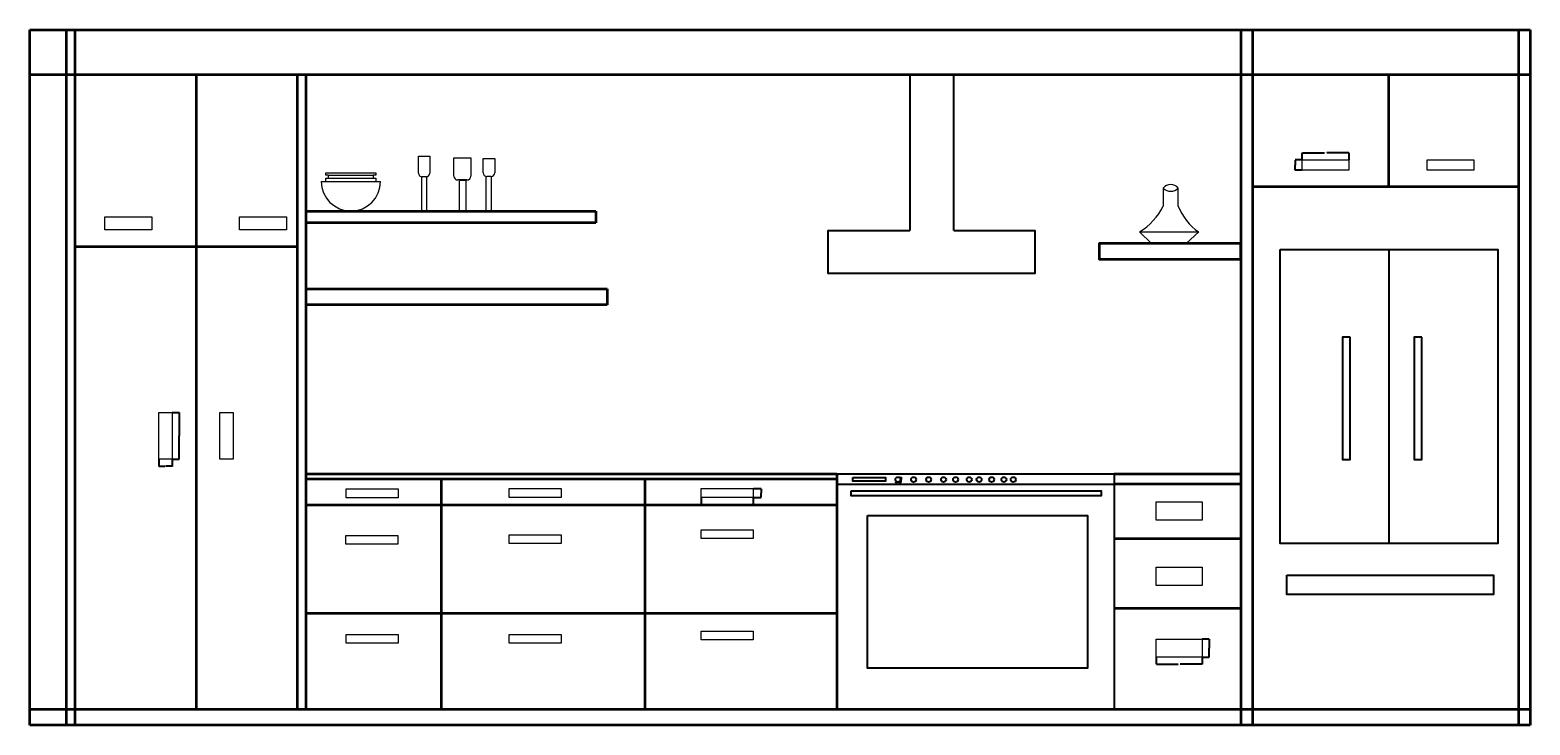
# Model space of a CAD drawing. Units: millimetres. Extents: x 3194 to 5786, y 875 to 2077.
import ezdxf

# ---------------------------------------------------------------- set-up
doc = ezdxf.new("R2010")
doc.units = ezdxf.units.MM
for name, color, linetype, lineweight in [('A-ANNO-DIMS', 2, 'Continuous', 18), ('A-ELEV', 7, 'Continuous', 35), ('A-ELEV-HRDW', 8, 'Continuous', 18), ('A-EQPM', 4, 'Continuous', 25), ('A-FURN', 9, 'Continuous', 18)]:
    doc.layers.add(name, color=color, linetype=linetype, lineweight=lineweight)
doc.styles.get("Standard").update_dxf_attribs({"font": 'arial.ttf'})
doc.dimstyles.get("Standard").update_dxf_attribs({"dimtxt": 0.18, "dimasz": 0.18, "dimexe": 0.18, "dimexo": 0.0625, "dimgap": 0.09, "dimtad": 0, "dimtih": 1, "dimtoh": 1, "dimdec": 4, "dimzin": 0, "dimdsep": 46, "dimtxsty": 'Standard', "dimcen": 0.09, "dimadec": 0, "dimazin": 0, "dimtfac": 1, "dimtdec": 4, "dimtofl": 0, "dimtmove": 0, "dimatfit": 3, "dimfxl": 1, "dimtolj": 1, "dimtzin": 0, "dimarcsym": 0})

# ---------------------------------------------------------------- blocks, each defined once
blk = doc.blocks.new('KNOB-RANGE')
blk.add_circle((4.3, 4.3), 4.31)
blk = doc.blocks.new('PULL-DRAWER-90')
blk.add_lwpolyline([(0, 15.2), (90, 15.2), (90, 0), (0, 0)], close=True)
blk = doc.blocks.new('PULL-DOOR-80')
blk.add_lwpolyline([(0, 81.1), (22.9, 81.1), (22.9, 0), (0, 0)], close=True)
blk = doc.blocks.new('PULL-DRAWER-80')
blk.add_lwpolyline([(0, 31.7), (79.4, 31.7), (79.4, 0), (0, 0)], close=True)
blk = doc.blocks.new('PULL-WALLCAB-80')
blk.add_lwpolyline([(0, 18), (80.8, 18), (80.8, 0), (0, 0)], close=True)
blk = doc.blocks.new('*D6')
at = {"layer": 'A-ANNO-DIMS', "color": 0, "lineweight": -2, "transparency": 16777216}
for p, q in [((4689.7, 1295.1), (4689.7, 1293.7)), ((4689.8, 1293.9), (4692.6, 1293.9)), ((4698.1, 1293.9), (4695.3, 1293.9)), ((4698.3, 1295.1), (4698.3, 1293.7))]:
    blk.add_line(p, q, dxfattribs=at)
at = {"layer": 'A-ANNO-DIMS', "color": 0, "transparency": 16777216}
for points in [[(4689.8, 1293.9), (4689.8, 1293.8), (4689.7, 1293.9)], [(4698.1, 1293.9), (4698.1, 1293.8), (4698.3, 1293.9)]]:
    blk.add_solid(points, dxfattribs=at)
at = {"layer": 'Defpoints', "color": 0, "transparency": 16777216}
for p in [(4689.7, 1295.2), (4698.3, 1295.2), (4698.3, 1293.9)]:
    blk.add_point(p, dxfattribs=at)
at = {"layer": 'A-ANNO-DIMS', "color": 0, "transparency": 16777216, "insert": (4694, 1293.9), "char_height": 0.18, "attachment_point": 5}
blk.add_mtext('\\A1;RANGE KNOB 9 TYP.', dxfattribs=at)
blk = doc.blocks.new('*D7')
at = {"layer": 'A-ANNO-DIMS', "color": 0, "lineweight": -2, "transparency": 16777216}
for p, q in [((4698.3, 1303.8), (4699.8, 1303.8)), ((4699.6, 1303.6), (4699.6, 1299.6)), ((4699.6, 1295.3), (4699.6, 1299.3)), ((4698.3, 1295.2), (4699.8, 1295.2))]:
    blk.add_line(p, q, dxfattribs=at)
at = {"layer": 'A-ANNO-DIMS', "color": 0, "transparency": 16777216}
for points in [[(4699.5, 1303.6), (4699.6, 1303.6), (4699.6, 1303.8)], [(4699.5, 1295.3), (4699.6, 1295.3), (4699.6, 1295.2)]]:
    blk.add_solid(points, dxfattribs=at)
at = {"layer": 'Defpoints', "color": 0, "transparency": 16777216}
for p in [(4698.3, 1303.8), (4699.6, 1303.8), (4698.3, 1295.2)]:
    blk.add_point(p, dxfattribs=at)
at = {"layer": 'A-ANNO-DIMS', "color": 0, "transparency": 16777216, "insert": (4699.6, 1299.5), "char_height": 0.18, "attachment_point": 5}
blk.add_mtext('\\A1;9 TYP.', dxfattribs=at)
blk = doc.blocks.new('*D8')
at = {"layer": 'A-ANNO-DIMS', "color": 0, "lineweight": -2, "transparency": 16777216}
for p, q in [((4354.1, 1268.6), (4354.1, 1254.9)), ((4354.3, 1255.1), (4397.6, 1255.1)), ((4443.9, 1255.1), (4400.6, 1255.1)), ((4444.1, 1268.6), (4444.1, 1254.9))]:
    blk.add_line(p, q, dxfattribs=at)
at = {"layer": 'A-ANNO-DIMS', "color": 0, "transparency": 16777216}
for points in [[(4354.3, 1255.2), (4354.3, 1255.1), (4354.1, 1255.1)], [(4443.9, 1255.2), (4443.9, 1255.1), (4444.1, 1255.1)]]:
    blk.add_solid(points, dxfattribs=at)
at = {"layer": 'Defpoints', "color": 0, "transparency": 16777216}
for p in [(4354.1, 1268.6), (4444.1, 1268.6), (4444.1, 1255.1)]:
    blk.add_point(p, dxfattribs=at)
at = {"layer": 'A-ANNO-DIMS', "color": 0, "transparency": 16777216, "insert": (4399.1, 1255.1), "char_height": 0.18, "attachment_point": 5}
blk.add_mtext('\\A1;DRAWER PULL 90 TYP.', dxfattribs=at)
blk = doc.blocks.new('*D9')
at = {"layer": 'A-ANNO-DIMS', "color": 0, "lineweight": -2, "transparency": 16777216}
for p, q in [((4444.2, 1283.9), (4457.8, 1283.9)), ((4457.6, 1283.7), (4457.6, 1276.4)), ((4457.6, 1268.8), (4457.6, 1276.1)), ((4444.2, 1268.6), (4457.8, 1268.6))]:
    blk.add_line(p, q, dxfattribs=at)
at = {"layer": 'A-ANNO-DIMS', "color": 0, "transparency": 16777216}
for points in [[(4457.6, 1283.7), (4457.6, 1283.7), (4457.6, 1283.9)], [(4457.6, 1268.8), (4457.6, 1268.8), (4457.6, 1268.6)]]:
    blk.add_solid(points, dxfattribs=at)
at = {"layer": 'Defpoints', "color": 0, "transparency": 16777216}
for p in [(4444.1, 1283.9), (4457.6, 1283.9), (4444.1, 1268.6)]:
    blk.add_point(p, dxfattribs=at)
at = {"layer": 'A-ANNO-DIMS', "color": 0, "transparency": 16777216, "insert": (4457.6, 1276.2), "char_height": 0.18, "attachment_point": 5}
blk.add_mtext('\\A1;15 TYP.', dxfattribs=at)
blk = doc.blocks.new('*D10')
at = {"layer": 'A-ANNO-DIMS', "color": 0, "lineweight": -2, "transparency": 16777216}
for p, q in [((5140.3, 992), (5140.3, 980)), ((5219.7, 992), (5219.7, 980)), ((5140.5, 980.1), (5178.1, 980.1)), ((5219.6, 980.1), (5181.9, 980.1))]:
    blk.add_line(p, q, dxfattribs=at)
at = {"layer": 'A-ANNO-DIMS', "color": 0, "transparency": 16777216}
for points in [[(5140.5, 980.2), (5140.5, 980.1), (5140.3, 980.1)], [(5219.6, 980.2), (5219.6, 980.1), (5219.7, 980.1)]]:
    blk.add_solid(points, dxfattribs=at)
at = {"layer": 'Defpoints', "color": 0, "transparency": 16777216}
for p in [(5140.3, 992), (5219.7, 992), (5219.7, 980.1)]:
    blk.add_point(p, dxfattribs=at)
at = {"layer": 'A-ANNO-DIMS', "color": 0, "transparency": 16777216, "insert": (5180, 980.1), "char_height": 0.18, "attachment_point": 5}
blk.add_mtext('\\A1;SMALL DRAWER PULL 79 TYP.', dxfattribs=at)
blk = doc.blocks.new('*D11')
at = {"layer": 'A-ANNO-DIMS', "color": 0, "lineweight": -2, "transparency": 16777216}
for p, q in [((5219.8, 1023.8), (5231.8, 1023.8)), ((5231.7, 1023.6), (5231.7, 1008.1)), ((5219.8, 992), (5231.8, 992)), ((5231.7, 992.2), (5231.7, 1007.7))]:
    blk.add_line(p, q, dxfattribs=at)
at = {"layer": 'A-ANNO-DIMS', "color": 0, "transparency": 16777216}
for points in [[(5231.6, 1023.6), (5231.7, 1023.6), (5231.7, 1023.8)], [(5231.6, 992.2), (5231.7, 992.2), (5231.7, 992)]]:
    blk.add_solid(points, dxfattribs=at)
at = {"layer": 'Defpoints', "color": 0, "transparency": 16777216}
for p in [(5219.7, 1023.8), (5231.7, 1023.8), (5219.7, 992)]:
    blk.add_point(p, dxfattribs=at)
at = {"layer": 'A-ANNO-DIMS', "color": 0, "transparency": 16777216, "insert": (5231.7, 1007.9), "char_height": 0.18, "attachment_point": 5}
blk.add_mtext('\\A1;32 TYP.', dxfattribs=at)
blk = doc.blocks.new('*D12')
at = {"layer": 'A-ANNO-DIMS', "color": 0, "lineweight": -2, "transparency": 16777216}
for p, q in [((3439.9, 1415.7), (3452.2, 1415.7)), ((3452, 1415.5), (3452, 1375.3)), ((3452, 1334.8), (3452, 1375)), ((3439.9, 1334.6), (3452.2, 1334.6))]:
    blk.add_line(p, q, dxfattribs=at)
at = {"layer": 'A-ANNO-DIMS', "color": 0, "transparency": 16777216}
for points in [[(3452, 1415.5), (3452.1, 1415.5), (3452, 1415.7)], [(3452, 1334.8), (3452.1, 1334.8), (3452, 1334.6)]]:
    blk.add_solid(points, dxfattribs=at)
at = {"layer": 'Defpoints', "color": 0, "transparency": 16777216}
for p in [(3439.9, 1415.7), (3452, 1415.7), (3439.9, 1334.6)]:
    blk.add_point(p, dxfattribs=at)
at = {"layer": 'A-ANNO-DIMS', "color": 0, "transparency": 16777216, "insert": (3452, 1375.2), "char_height": 0.18, "attachment_point": 5}
blk.add_mtext('\\A1;TALL DOOR PULL 81 TYP.', dxfattribs=at)
blk = doc.blocks.new('*D13')
at = {"layer": 'A-ANNO-DIMS', "color": 0, "lineweight": -2, "transparency": 16777216}
for p, q in [((3417, 1334.5), (3417, 1322.3)), ((3417.2, 1322.4), (3427.9, 1322.4)), ((3439.7, 1322.4), (3429, 1322.4)), ((3439.9, 1334.5), (3439.9, 1322.3))]:
    blk.add_line(p, q, dxfattribs=at)
at = {"layer": 'A-ANNO-DIMS', "color": 0, "transparency": 16777216}
for points in [[(3417.2, 1322.5), (3417.2, 1322.4), (3417, 1322.4)], [(3439.7, 1322.5), (3439.7, 1322.4), (3439.9, 1322.4)]]:
    blk.add_solid(points, dxfattribs=at)
at = {"layer": 'Defpoints', "color": 0, "transparency": 16777216}
for p in [(3417, 1334.6), (3439.9, 1334.6), (3439.9, 1322.4)]:
    blk.add_point(p, dxfattribs=at)
at = {"layer": 'A-ANNO-DIMS', "color": 0, "transparency": 16777216, "insert": (3428.4, 1322.4), "char_height": 0.18, "attachment_point": 5}
blk.add_mtext('\\A1;23 TYP.', dxfattribs=at)
blk = doc.blocks.new('*D14')
at = {"layer": 'A-ANNO-DIMS', "color": 0, "lineweight": -2, "transparency": 16777216}
for p, q in [((5392.6, 1852.5), (5392.6, 1864.7)), ((5392.8, 1864.6), (5431.2, 1864.6)), ((5473.3, 1864.6), (5434.9, 1864.6)), ((5473.5, 1852.5), (5473.5, 1864.7))]:
    blk.add_line(p, q, dxfattribs=at)
at = {"layer": 'A-ANNO-DIMS', "color": 0, "transparency": 16777216}
for points in [[(5392.8, 1864.6), (5392.8, 1864.5), (5392.6, 1864.6)], [(5473.3, 1864.6), (5473.3, 1864.5), (5473.5, 1864.6)]]:
    blk.add_solid(points, dxfattribs=at)
at = {"layer": 'Defpoints', "color": 0, "transparency": 16777216}
for p in [(5392.6, 1852.4), (5473.5, 1864.6), (5473.5, 1852.4)]:
    blk.add_point(p, dxfattribs=at)
at = {"layer": 'A-ANNO-DIMS', "color": 0, "transparency": 16777216, "insert": (5433.1, 1864.6), "char_height": 0.18, "attachment_point": 5}
blk.add_mtext('\\A1;WALL CABINET PULL 81 TYP.', dxfattribs=at)
blk = doc.blocks.new('*D15')
at = {"layer": 'A-ANNO-DIMS', "color": 0, "lineweight": -2, "transparency": 16777216}
for p, q in [((5392.6, 1852.4), (5380.3, 1852.4)), ((5380.5, 1852.2), (5380.5, 1843.6)), ((5380.5, 1834.7), (5380.5, 1843.3)), ((5392.6, 1834.5), (5380.3, 1834.5))]:
    blk.add_line(p, q, dxfattribs=at)
at = {"layer": 'A-ANNO-DIMS', "color": 0, "transparency": 16777216}
for points in [[(5380.5, 1852.2), (5380.5, 1852.2), (5380.5, 1852.4)], [(5380.5, 1834.7), (5380.5, 1834.7), (5380.5, 1834.5)]]:
    blk.add_solid(points, dxfattribs=at)
at = {"layer": 'Defpoints', "color": 0, "transparency": 16777216}
for p in [(5380.5, 1852.4), (5392.6, 1852.4), (5392.6, 1834.5)]:
    blk.add_point(p, dxfattribs=at)
at = {"layer": 'A-ANNO-DIMS', "color": 0, "transparency": 16777216, "insert": (5380.5, 1843.4), "char_height": 0.18, "attachment_point": 5}
blk.add_mtext('\\A1;18 TYP.', dxfattribs=at)

msp = doc.modelspace()

# ---------------------------------------------------------------- linework, layer by layer
at = {"layer": 'A-ELEV'}
for p, q in [((3194.2, 2077.2), (5786.2, 2077.2)), ((3194.2, 874.9), (3194.2, 2077.2)), ((3256.7, 2077.2), (3256.7, 874.9)), ((3271.7, 2077.2), (3271.7, 874.9)), ((5286.7, 2077.2), (5286.7, 874.9)), ((5306.7, 2077.2), (5306.7, 874.9)), ((5766.2, 2077.2), (5766.2, 874.9)), ((5786.2, 2077.2), (5786.2, 874.9)), ((3194.2, 2000.2), (5786.2, 2000.2)), ((3481.5, 2000.2), (3481.5, 901.9)), ((3656, 2000.2), (3656, 901.9)), ((3671, 2000.2), (3671, 901.9)), ((5542.3, 1806), (5542.3, 2000.2)), ((5766.2, 1806), (5306.7, 1806)), ((3671, 1764), (4172.2, 1764)), ((4172.2, 1764), (4172.2, 1743.8)), ((4172.2, 1743.8), (3671, 1743.8)), ((3271.7, 1702.8), (3656, 1702.8)), ((3671, 1629.6), (4191.7, 1629.6)), ((4191.7, 1629.6), (4191.7, 1601.6)), ((4191.7, 1601.6), (3671, 1601.6)), ((3671, 1309.4), (4588.4, 1309.4)), ((4588.4, 1300.4), (3671, 1300.4)), ((3904.9, 1300.4), (3904.9, 901.9)), ((4256.8, 1300.4), (4256.8, 901.9)), ((4588.4, 1309.4), (4588.4, 901.9)), ((5067.6, 1309.4), (5286.7, 1309.4)), ((5286.7, 1309.4), (5286.7, 1291.4)), ((5286.7, 1291.4), (5067.6, 1291.4)), ((4588.4, 1255.4), (3671, 1255.4)), ((5067.6, 1197.4), (5286.7, 1197.4)), ((5286.7, 1197.4), (5286.7, 1076.4)), ((4588.4, 1067.7), (3671, 1067.7)), ((5286.7, 1076.4), (5067.6, 1076.4)), ((5786.2, 901.9), (3194.2, 901.9)), ((5786.2, 874.9), (3194.2, 874.9))]:
    msp.add_line(p, q, dxfattribs=at)
msp.add_lwpolyline([(5286.7, 1707.6), (5041.5, 1707.6), (5041.5, 1680.6), (5286.7, 1680.6)], close=True, dxfattribs=at)
at = {"layer": 'A-EQPM'}
for p, q in [((5542.3, 1697.7), (5542.3, 1188.8)), ((4588.4, 1291.4), (5067.6, 1291.4))]:
    msp.add_line(p, q, dxfattribs=at)
for points in [[(4790.5, 1730.5), (4790.5, 2000.2), (4714.6, 2000.2), (4714.6, 1730.5)], [(4790.5, 1730.5), (4930.4, 1730.5), (4930.4, 1656.2), (4573.3, 1656.2), (4573.3, 1730.5), (4714.6, 1730.5)], [(5599.2, 1545.9), (5585.8, 1545.9)], [(5585.8, 1334.2), (5599.2, 1334.2)]]:
    msp.add_lwpolyline(points, dxfattribs=at)
for points in [[(5354.3, 1697.7), (5730.3, 1697.7), (5730.3, 1188.8), (5354.3, 1188.8)], [(5475.3, 1545.9), (5461.9, 1545.9), (5461.9, 1334.2), (5475.3, 1334.2)], [(5599.2, 1545.9), (5585.8, 1545.9), (5585.8, 1334.2), (5599.2, 1334.2)], [(4588.4, 1309.4), (5067.6, 1309.4), (5067.6, 901.9), (4588.4, 901.9)], [(4616, 1302.8), (4672.5, 1302.8), (4672.5, 1296.7), (4616, 1296.7)], [(4613.3, 1279.8), (5045.2, 1279.8), (5045.2, 1271.3), (4613.3, 1271.3)], [(4641.3, 1237.3), (5021.5, 1237.3), (5021.5, 973.4), (4641.3, 973.4)], [(5366.2, 1134.1), (5723.2, 1134.1), (5723.2, 1100.8), (5366.2, 1100.8)]]:
    msp.add_lwpolyline(points, close=True, dxfattribs=at)
at = {"layer": 'A-FURN'}
for p, q in [((3865.6, 1859), (3884.9, 1859)), ((3865.6, 1829.7), (3865.6, 1859)), ((3884.9, 1859), (3884.9, 1829.7)), ((3926.8, 1856.3), (3955.9, 1856.3)), ((3926.8, 1824.3), (3926.8, 1856.3)), ((3955.9, 1856.3), (3955.9, 1824.3)), ((3977.2, 1854.9), (3997.2, 1854.9)), ((3977.2, 1830.1), (3977.2, 1854.9)), ((3997.2, 1854.9), (3997.2, 1830.1)), ((3697.6, 1815.1), (3799.8, 1815.1)), ((3705.6, 1826), (3705.6, 1830.3)), ((3705.6, 1830.3), (3791.7, 1830.3)), ((3709.9, 1826), (3705.6, 1826)), ((3705.6, 1815.1), (3705.6, 1821.1)), ((3705.6, 1821.1), (3791.7, 1821.1)), ((3709.9, 1821.1), (3709.9, 1826)), ((3709.9, 1826), (3787.3, 1826)), ((3787.3, 1826), (3787.3, 1821.1)), ((3791.7, 1826), (3787.3, 1826)), ((3791.7, 1830.3), (3791.7, 1826)), ((3791.7, 1821.1), (3791.7, 1815.1)), ((3871.1, 1823.5), (3879.1, 1823.5)), ((3871.1, 1763.9), (3871.1, 1823.5)), ((3878.3, 1823.1), (3872.2, 1823.1)), ((3879.1, 1823.5), (3879.1, 1763.9)), ((3949.3, 1817.7), (3933.4, 1817.7)), ((3936.3, 1817.6), (3947.1, 1817.6)), ((3936.3, 1763.9), (3936.3, 1817.6)), ((3947.1, 1817.6), (3947.1, 1763.9)), ((3982.7, 1763.9), (3982.7, 1823.5)), ((3990.6, 1823.5), (3983.8, 1823.5)), ((3991.3, 1823.5), (3991.3, 1763.9)), ((5152.5, 1803.5), (5152.5, 1772.6)), ((5178.4, 1772.6), (5178.4, 1803.5)), ((5132.1, 1707.6), (5111.3, 1727.8)), ((5111.3, 1727.8), (5213.8, 1727.8)), ((5213.8, 1727.8), (5192.1, 1707.6))]:
    msp.add_line(p, q, dxfattribs=at)
for centre, radius, start, end in [((3748.7, 1815.1), 51.1, 180, 0), ((3872.2, 1829.7), 6.59, 180, 270), ((3878.3, 1829.7), 6.59, 270, 0), ((3933.4, 1824.3), 6.59, 180, 270), ((3949.3, 1824.3), 6.59, 270, 0), ((3983.8, 1830.1), 6.59, 180, 270), ((3990.6, 1830.1), 6.59, 270, 0), ((5165.4, 1793.6), 16.3, 37.4533, 142.5467), ((5165.4, 1816.9), 18.6, 225.8486, 314.1514), ((5052.9, 1822.9), 111.5, 301.5814, 333.1995), ((5267.6, 1806.5), 95.5, 200.7998, 235.564)]:
    msp.add_arc(centre, radius, start, end, dxfattribs=at)

# ---------------------------------------------------------------- block references
at = {"layer": 'A-ELEV-HRDW'}
for name, p in [('PULL-WALLCAB-80', (5392.6, 1834.5)), ('PULL-WALLCAB-80', (5608.2, 1834.5)), ('PULL-DOOR-80', (3417, 1334.6)), ('PULL-DOOR-80', (3522.1, 1334.6)), ('PULL-DRAWER-90', (3740.3, 1268.1)), ('PULL-DRAWER-90', (4022.3, 1268.6)), ('PULL-DRAWER-90', (4354.1, 1268.6)), ('PULL-DRAWER-80', (5140.3, 1229.2)), ('PULL-DRAWER-90', (3740.1, 1187.8)), ('PULL-DRAWER-90', (4022.3, 1188.9)), ('PULL-DRAWER-90', (4354.1, 1197.4)), ('PULL-DRAWER-80', (5140.3, 1116.1)), ('PULL-DRAWER-90', (4354.1, 1022.2)), ('PULL-DRAWER-90', (3740.3, 1016.3)), ('PULL-DRAWER-90', (4022.3, 1016.3)), ('PULL-DRAWER-80', (5140.3, 992))]:
    msp.add_blockref(name, p, dxfattribs=at)
for p, rotation in [((3323.4, 1754.2), 269.9999999999998), ((3556.5, 1754.2), 270)]:
    msp.add_blockref('PULL-DOOR-80', p, dxfattribs=dict(at, rotation=rotation))
at = {"layer": 'A-EQPM'}
for p in [(4689.7, 1295.1), (4716.7, 1295.1), (4742.8, 1295.1), (4768.5, 1295.1), (4789.3, 1295.1), (4812.8, 1295.1), (4830, 1295.1), (4851.6, 1295.1), (4872.7, 1295.1), (4889, 1295.1)]:
    msp.add_blockref('KNOB-RANGE', p, dxfattribs=at)

# ---------------------------------------------------------------- dimensions: what is measured, and where the dimension line sits
at = {"layer": 'A-ANNO-DIMS'}
for base, p1, p2, text, picture, middle in [((5380.5, 1852.4), (5392.6, 1834.5), (5392.6, 1852.4), '<> TYP.', '*D15', (5380.5, 1843.4)), ((3452, 1415.7), (3439.9, 1334.6), (3439.9, 1415.7), 'TALL DOOR PULL <> TYP.', '*D12', (3452, 1375.2)), ((4699.6, 1303.8), (4698.3, 1295.1), (4698.3, 1303.8), '<> TYP.', '*D7', (4699.6, 1299.5)), ((4457.6, 1283.9), (4444.1, 1268.6), (4444.1, 1283.9), '<> TYP.', '*D9', (4457.6, 1276.2)), ((5231.7, 1023.8), (5219.7, 992), (5219.7, 1023.8), '<> TYP.', '*D11', (5231.7, 1007.9))]:
    dim = msp.add_linear_dim(base=base, p1=p1, p2=p2, angle=90, text=text, dimstyle='Standard', override={"dimdec": 0, "dimrnd": 0, "dimzin": 0, "dimlunit": 2}, dxfattribs=at)
    dim.commit()
    dim.dimension.update_dxf_attribs({"geometry": picture, "text_midpoint": middle})
for base, p1, p2, text, picture, middle in [((5473.5, 1864.6), (5392.6, 1852.4), (5473.5, 1852.4), 'WALL CABINET PULL <> TYP.', '*D14', (5433.1, 1864.6)), ((3439.9, 1322.4), (3417, 1334.6), (3439.9, 1334.6), '<> TYP.', '*D13', (3428.4, 1322.4)), ((4698.3, 1293.9), (4689.7, 1295.1), (4698.3, 1295.1), 'RANGE KNOB <> TYP.', '*D6', (4694, 1293.9)), ((4444.1, 1255.1), (4354.1, 1268.6), (4444.1, 1268.6), 'DRAWER PULL <> TYP.', '*D8', (4399.1, 1255.1)), ((5219.7, 980.1), (5140.3, 992), (5219.7, 992), 'SMALL DRAWER PULL <> TYP.', '*D10', (5180, 980.1))]:
    dim = msp.add_linear_dim(base=base, p1=p1, p2=p2, text=text, dimstyle='Standard', override={"dimdec": 0, "dimrnd": 0, "dimzin": 0, "dimlunit": 2}, dxfattribs=at)
    dim.commit()
    dim.dimension.update_dxf_attribs({"geometry": picture, "text_midpoint": middle})

doc.saveas('drawing.dxf')
